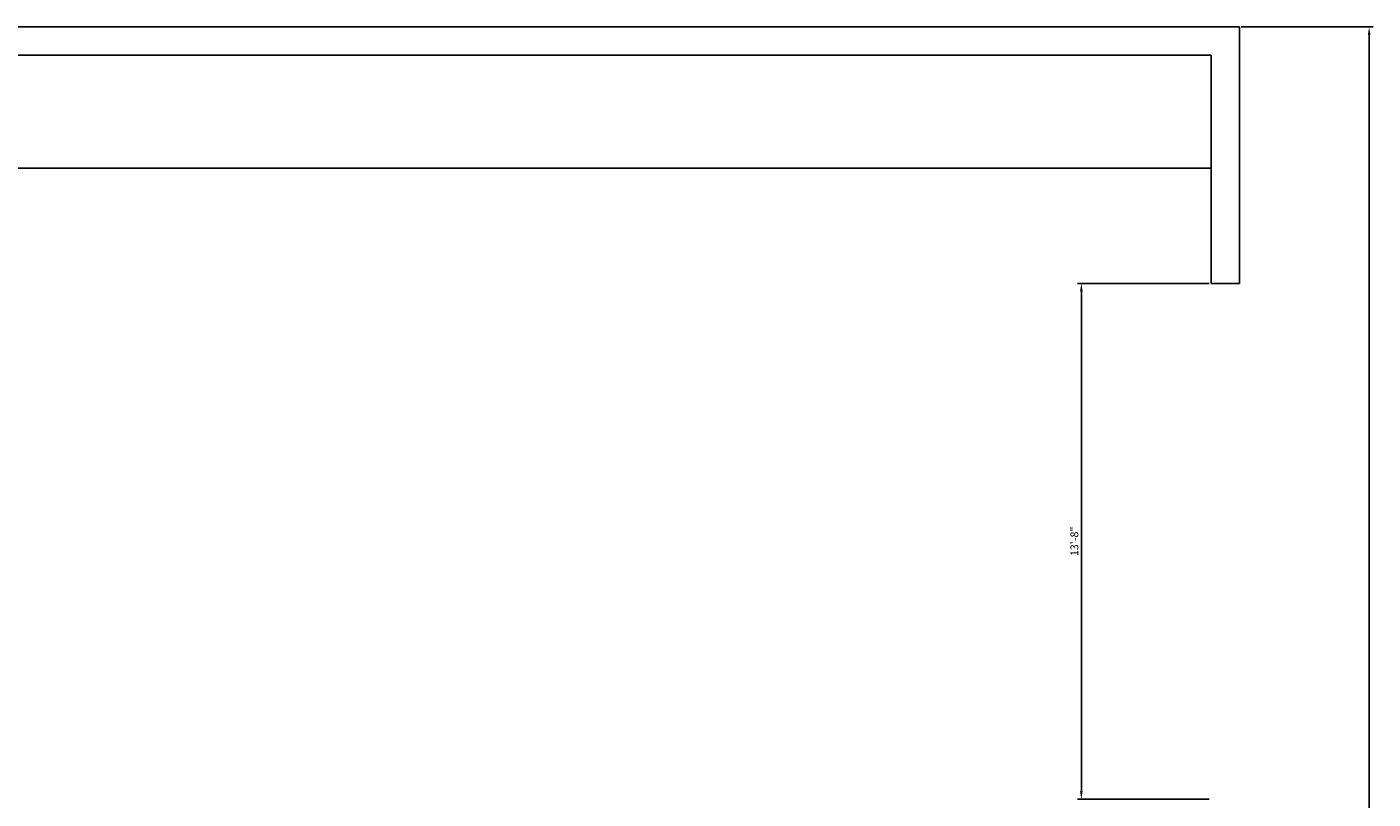
# Model space of a CAD drawing. Units: inches. Extents: x 250205121 to 250208111, y 89832590 to 89833271.
# Tile 4 of 14: x 250205601 to 250206030, y 89832978 to 89833224. Entities that reach past the tile are written whole.
import ezdxf

# ---------------------------------------------------------------- set-up
doc = ezdxf.new("R2010")
doc.units = ezdxf.units.IN
doc.layers.add('C-PROP', color=8, linetype='Continuous', lineweight=25)
doc.layers.add('dimensions', color=2, linetype='Continuous', lineweight=18)
doc.styles.get("Standard").update_dxf_attribs({"font": 'arial.ttf'})
doc.dimstyles.new('ISO-25', dxfattribs={"dimtxt": 2.5, "dimasz": 2.5, "dimexe": 1.25, "dimexo": 0.625, "dimtad": 1, "dimlunit": 4, "dimtxsty": 'Standard', "dimcen": 2.5, "dimadec": 0, "dimazin": 0, "dimtfac": 1, "dimtmove": 0, "dimatfit": 3, "dimfxl": 1, "dimarcsym": 0})

# ---------------------------------------------------------------- blocks, each defined once
blk = doc.blocks.new('*D42')
at = {"layer": 'Defpoints', "color": 0, "transparency": 16777216}
for p in [(250205986.91, 89833224.33), (250206028.26, 89833224.33), (250205986.91, 89832633.33)]:
    blk.add_point(p, dxfattribs=at)
at = {"layer": 'dimensions', "color": 0, "lineweight": -2, "transparency": 16777216}
for p, q in [((250205987.53, 89833224.33), (250206029.51, 89833224.33)), ((250206028.26, 89832635.83), (250206028.26, 89833221.83)), ((250205987.53, 89832633.33), (250206029.51, 89832633.33))]:
    blk.add_line(p, q, dxfattribs=at)
at = {"layer": 'dimensions', "color": 0, "transparency": 16777216}
for points in [[(250206027.84, 89833221.83), (250206028.67, 89833221.83), (250206028.26, 89833224.33)], [(250206027.84, 89832635.83), (250206028.67, 89832635.83), (250206028.26, 89832633.33)]]:
    blk.add_solid(points, dxfattribs=at)
at = {"layer": 'dimensions', "color": 0, "transparency": 16777216, "insert": (250206026.36, 89832928.83), "char_height": 2.5, "attachment_point": 5, "rotation": 90}
blk.add_mtext('49\'-3"', dxfattribs=at)
blk = doc.blocks.new('*D49')
at = {"layer": 'Defpoints', "color": 0, "transparency": 16777216}
for p in [(250205936.56, 89833142.57), (250205977.91, 89833142.57), (250205977.91, 89832978.33)]:
    blk.add_point(p, dxfattribs=at)
at = {"layer": 'dimensions', "color": 0, "lineweight": -2, "transparency": 16777216}
for p, q in [((250205977.28, 89833142.57), (250205935.31, 89833142.57)), ((250205936.56, 89832980.83), (250205936.56, 89833140.07)), ((250205977.28, 89832978.33), (250205935.31, 89832978.33))]:
    blk.add_line(p, q, dxfattribs=at)
at = {"layer": 'dimensions', "color": 0, "transparency": 16777216}
for points in [[(250205936.14, 89833140.07), (250205936.97, 89833140.07), (250205936.56, 89833142.57)], [(250205936.14, 89832980.83), (250205936.97, 89832980.83), (250205936.56, 89832978.33)]]:
    blk.add_solid(points, dxfattribs=at)
at = {"layer": 'dimensions', "color": 0, "transparency": 16777216, "insert": (250205934.66, 89833060.45), "char_height": 2.5, "attachment_point": 5, "rotation": 90}
blk.add_mtext('13\'-8"', dxfattribs=at)

msp = doc.modelspace()

# ---------------------------------------------------------------- linework, layer by layer
at = {"layer": 'C-PROP'}
for p, q in [((250205500.908, 89833224.328), (250205977.908, 89833224.328)), ((250205977.908, 89833224.328), (250205986.908, 89833224.328)), ((250205986.908, 89833224.328), (250205986.908, 89833178.574)), ((250205977.908, 89833215.328), (250205500.908, 89833215.328)), ((250205977.908, 89833179.328), (250205977.908, 89833215.328)), ((250205509.908, 89833179.328), (250205680.908, 89833179.328)), ((250205680.908, 89833179.328), (250205689.908, 89833179.328)), ((250205689.908, 89833179.328), (250205800.908, 89833179.328)), ((250205800.908, 89833179.328), (250205805.408, 89833179.328)), ((250205805.408, 89833179.328), (250205905.908, 89833179.328)), ((250205905.908, 89833179.328), (250205977.908, 89833179.328)), ((250205977.908, 89833142.574), (250205977.908, 89833179.328)), ((250205986.908, 89833178.574), (250205986.908, 89833142.574)), ((250205986.908, 89833142.574), (250205977.908, 89833142.574))]:
    msp.add_line(p, q, dxfattribs=at)

# ---------------------------------------------------------------- dimensions: what is measured, and where the dimension line sits
at = {"layer": 'dimensions'}
for base, p1, p2, picture, middle in [((250206028.258, 89833224.328), (250205986.908, 89832633.328), (250205986.908, 89833224.328), '*D42', (250206026.355, 89832928.828)), ((250205936.558, 89833142.574), (250205977.908, 89832978.328), (250205977.908, 89833142.574), '*D49', (250205934.655, 89833060.451))]:
    dim = msp.add_linear_dim(base=base, p1=p1, p2=p2, angle=90, dimstyle='ISO-25', override={"dimdec": 1, "dimlfac": 1, "dimrnd": 0, "dimzin": 1, "dimdsep": 46, "dimlunit": 4, "dimfrac": 2}, dxfattribs=at)
    dim.commit()
    dim.dimension.update_dxf_attribs({"geometry": picture, "text_midpoint": middle})

doc.saveas('drawing.dxf')
